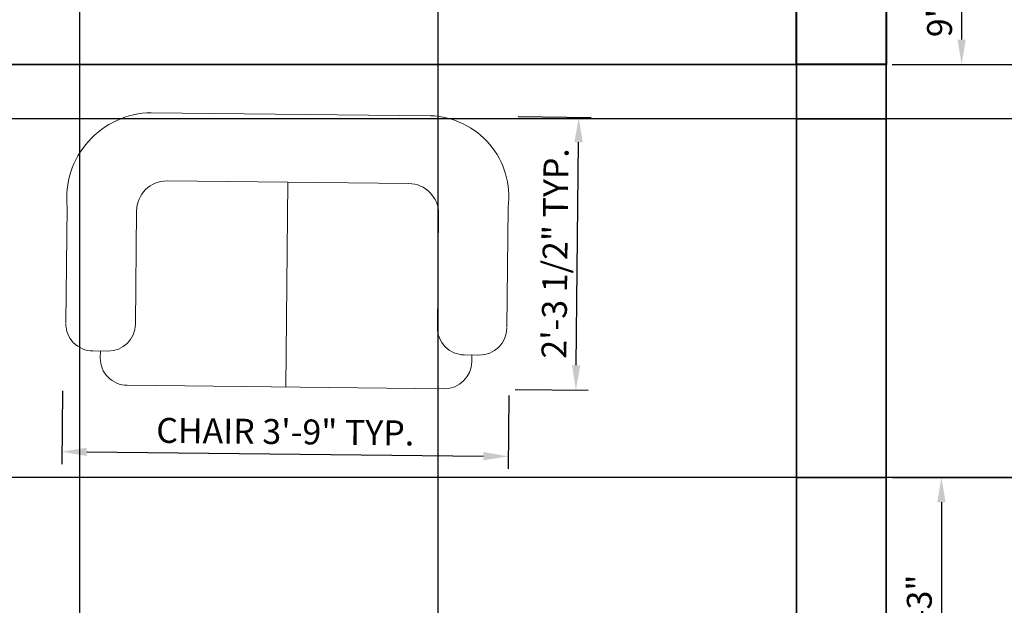
# Model space of a CAD drawing. Units: inches. Extents: x 1624 to 3956, y 1589 to 5028.
# Tile 7 of 16: x 2014 to 2112, y 2191 to 2250. Entities that reach past the tile are written whole.
import ezdxf

# ---------------------------------------------------------------- set-up
doc = ezdxf.new("R2010")
doc.units = ezdxf.units.IN
for name, color, linetype, lineweight in [('A-ANNO-DIMS', 2, 'Continuous', 13), ('A-COLS', 1, 'Continuous', 40), ('A-FURN', 8, 'Continuous', 18), ('A-WALL', 7, 'Continuous', 35)]:
    doc.layers.add(name, color=color, linetype=linetype, lineweight=lineweight)
doc.styles.get("Standard").update_dxf_attribs({"font": 'arial.ttf'})
doc.dimstyles.new('Copy of ISO-25', dxfattribs={"dimtxt": 2.5, "dimasz": 2.5, "dimexe": 1.25, "dimexo": 0.625, "dimtad": 1, "dimdec": 1, "dimlunit": 4, "dimtxsty": 'Standard', "dimcen": 2.5, "dimadec": 0, "dimazin": 0, "dimtfac": 1, "dimtdec": 1, "dimtmove": 0, "dimatfit": 3, "dimfxl": 1, "dimarcsym": 0})

# ---------------------------------------------------------------- blocks, each defined once
blk = doc.blocks.new('A$C6D011943')
for p, q in [((1.4484, 1.0893), (0.3319, 1.0893)), ((1.3639, 0.8177), (0.3983, 0.8177)), ((0.8811, 0.8177), (0.8811, 0)), ((0, 0.7091), (0, 0.2474)), ((1.7622, 0.2474), (1.7622, 0.7272)), ((0.2776, 0.697), (0.2776, 0.2444)), ((1.4846, 0.2444), (1.4846, 0.697)), ((0.1086, 0.1358), (0.169, 0.1358)), ((0.1388, 0.1086), (0.1388, 0.1358)), ((1.5932, 0.1358), (1.6536, 0.1358)), ((1.6475, 0.1358), (1.6234, 0.1358)), ((1.6234, 0.1086), (1.6234, 0.1358)), ((1.5148, 0), (0.2474, 0))]:
    blk.add_line(p, q)
for centre, radius, start, end in [((0.3394, 0.7478), 0.3416, 91.2564, 186.501), ((1.4409, 0.7658), 0.3236, 353.159, 88.6697), ((0.3983, 0.697), 0.1207, 90, 180), ((1.3639, 0.697), 0.1207, 0, 90), ((0.1086, 0.2444), 0.1086, 180, 270), ((0.169, 0.2444), 0.1086, 270, 0), ((1.5932, 0.2444), 0.1086, 180, 270), ((1.6536, 0.2444), 0.1086, 270, 0), ((0.2474, 0.1086), 0.1086, 180, 270), ((1.5148, 0.1086), 0.1086, 270, 0)]:
    blk.add_arc(centre, radius, start, end)
blk = doc.blocks.new('*D38')
at = {"layer": 'A-ANNO-DIMS', "color": 0, "lineweight": -2, "transparency": 16777216}
for p, q in [((2101.204, 2254.295), (2109.428, 2254.295)), ((2108.178, 2251.795), (2108.178, 2247.795)), ((2101.204, 2245.295), (2109.428, 2245.295))]:
    blk.add_line(p, q, dxfattribs=at)
at = {"layer": 'A-ANNO-DIMS', "color": 0, "transparency": 16777216}
for points in [[(2107.761, 2251.795), (2108.594, 2251.795), (2108.178, 2254.295)], [(2107.761, 2247.795), (2108.594, 2247.795), (2108.178, 2245.295)]]:
    blk.add_solid(points, dxfattribs=at)
at = {"layer": 'Defpoints', "color": 0, "transparency": 16777216}
for p in [(2100.579, 2254.295), (2100.579, 2245.295), (2108.178, 2245.295)]:
    blk.add_point(p, dxfattribs=at)
at = {"layer": 'A-ANNO-DIMS', "color": 0, "transparency": 16777216, "insert": (2106.276, 2249.795), "char_height": 2.5, "attachment_point": 5, "rotation": 90}
blk.add_mtext('9"', dxfattribs=at)
blk = doc.blocks.new('*D39')
at = {"layer": 'A-ANNO-DIMS', "color": 0, "lineweight": -2, "transparency": 16777216}
for p, q in [((2101.204, 2203.835), (2107.397, 2203.835)), ((2106.147, 2201.335), (2106.147, 2179.295)), ((2101.204, 2176.795), (2107.397, 2176.795))]:
    blk.add_line(p, q, dxfattribs=at)
at = {"layer": 'A-ANNO-DIMS', "color": 0, "transparency": 16777216}
for points in [[(2105.73, 2201.335), (2106.564, 2201.335), (2106.147, 2203.835)], [(2105.73, 2179.295), (2106.564, 2179.295), (2106.147, 2176.795)]]:
    blk.add_solid(points, dxfattribs=at)
at = {"layer": 'Defpoints', "color": 0, "transparency": 16777216}
for p in [(2100.579, 2203.835), (2100.579, 2176.795), (2106.147, 2176.795)]:
    blk.add_point(p, dxfattribs=at)
at = {"layer": 'A-ANNO-DIMS', "color": 0, "transparency": 16777216, "insert": (2104.245, 2190.315), "char_height": 2.5, "attachment_point": 5, "rotation": 90}
blk.add_mtext('2\'-3"', dxfattribs=at)
blk = doc.blocks.new('COLUMN-9x9')
for p, q in [((0, 0), (0, 9)), ((0, 9), (9, 9)), ((9, 9), (9, 0)), ((9, 0), (0, 0))]:
    blk.add_line(p, q)
blk = doc.blocks.new('*D52')
at = {"layer": 'A-ANNO-DIMS', "color": 0, "lineweight": -2, "transparency": 16777216}
for p, q in [((2017.817, 2212.527), (2017.739, 2205.174)), ((2062.676, 2212.049), (2062.598, 2204.695)), ((2020.252, 2206.397), (2060.111, 2205.972))]:
    blk.add_line(p, q, dxfattribs=at)
at = {"layer": 'A-ANNO-DIMS', "color": 0, "transparency": 16777216}
for points in [[(2020.256, 2206.813), (2020.247, 2205.98), (2017.752, 2206.423)], [(2060.116, 2206.388), (2060.107, 2205.555), (2062.611, 2205.945)]]:
    blk.add_solid(points, dxfattribs=at)
at = {"layer": 'Defpoints', "color": 0, "transparency": 16777216}
for p in [(2017.824, 2213.152), (2062.683, 2212.674), (2062.611, 2205.945)]:
    blk.add_point(p, dxfattribs=at)
at = {"layer": 'A-ANNO-DIMS', "color": 0, "transparency": 16777216, "insert": (2040.202, 2208.103), "char_height": 2.5, "attachment_point": 5, "rotation": 359.38916}
blk.add_mtext('CHAIR 3\'-9" TYP.', dxfattribs=at)
blk = doc.blocks.new('*D53')
at = {"layer": 'A-ANNO-DIMS', "color": 0, "lineweight": -2, "transparency": 16777216}
for p, q in [((2063.6, 2240.059), (2070.954, 2239.981)), ((2069.438, 2215.102), (2069.677, 2237.495)), ((2063.308, 2212.667), (2070.662, 2212.589))]:
    blk.add_line(p, q, dxfattribs=at)
at = {"layer": 'A-ANNO-DIMS', "color": 0, "transparency": 16777216}
for points in [[(2069.26, 2237.499), (2070.094, 2237.49), (2069.704, 2239.994)], [(2069.022, 2215.107), (2069.855, 2215.098), (2069.412, 2212.602)]]:
    blk.add_solid(points, dxfattribs=at)
at = {"layer": 'Defpoints', "color": 0, "transparency": 16777216}
for p in [(2062.975, 2240.066), (2069.704, 2239.994), (2062.683, 2212.674)]:
    blk.add_point(p, dxfattribs=at)
at = {"layer": 'A-ANNO-DIMS', "color": 0, "transparency": 16777216, "insert": (2067.639, 2226.319), "char_height": 2.5, "attachment_point": 5, "rotation": 89.38916}
blk.add_mtext('2\'-3 1/2" TYP.', dxfattribs=at)
blk = doc.blocks.new('*D80')
at = {"layer": 'A-ANNO-DIMS', "color": 0, "lineweight": -2, "transparency": 16777216}
for p, q in [((2101.204, 2245.295), (2217.629, 2245.295)), ((2216.379, 2206.335), (2216.379, 2242.795)), ((2101.204, 2203.835), (2217.629, 2203.835))]:
    blk.add_line(p, q, dxfattribs=at)
at = {"layer": 'A-ANNO-DIMS', "color": 0, "transparency": 16777216}
for points in [[(2215.963, 2242.795), (2216.796, 2242.795), (2216.379, 2245.295)], [(2215.963, 2206.335), (2216.796, 2206.335), (2216.379, 2203.835)]]:
    blk.add_solid(points, dxfattribs=at)
at = {"layer": 'Defpoints', "color": 0, "transparency": 16777216}
for p in [(2100.579, 2245.295), (2216.379, 2245.295), (2100.579, 2203.835)]:
    blk.add_point(p, dxfattribs=at)
at = {"layer": 'A-ANNO-DIMS', "color": 0, "transparency": 16777216, "insert": (2214.461, 2224.565), "char_height": 2.5, "attachment_point": 5, "rotation": 90}
blk.add_mtext('3\'-5 1/2"', dxfattribs=at)
blk = doc.blocks.new('*D90')
at = {"layer": 'A-ANNO-DIMS', "color": 0, "lineweight": -2, "transparency": 16777216}
for p, q in [((2019.579, 1941.92), (2019.579, 2612.845)), ((2055.579, 1941.92), (2055.579, 2612.845)), ((2022.079, 2611.595), (2053.079, 2611.595))]:
    blk.add_line(p, q, dxfattribs=at)
at = {"layer": 'A-ANNO-DIMS', "color": 0, "transparency": 16777216}
for points in [[(2022.079, 2612.011), (2022.079, 2611.178), (2019.579, 2611.595)], [(2053.079, 2612.011), (2053.079, 2611.178), (2055.579, 2611.595)]]:
    blk.add_solid(points, dxfattribs=at)
at = {"layer": 'Defpoints', "color": 0, "transparency": 16777216}
for p in [(2055.579, 2611.595), (2019.579, 1941.295), (2055.579, 1941.295)]:
    blk.add_point(p, dxfattribs=at)
at = {"layer": 'A-ANNO-DIMS', "color": 0, "transparency": 16777216, "insert": (2037.579, 2613.497), "char_height": 2.5, "attachment_point": 5}
blk.add_mtext('3\'-0"', dxfattribs=at)
blk = doc.blocks.new('*D95')
at = {"layer": 'A-ANNO-DIMS', "color": 0, "lineweight": -2, "transparency": 16777216}
for p, q in [((1870.181, 2239.871), (2217.629, 2239.871)), ((2216.379, 2206.371), (2216.379, 2237.371)), ((1870.181, 2203.871), (2217.629, 2203.871))]:
    blk.add_line(p, q, dxfattribs=at)
at = {"layer": 'A-ANNO-DIMS', "color": 0, "transparency": 16777216}
for points in [[(2215.963, 2237.371), (2216.796, 2237.371), (2216.379, 2239.871)], [(2215.963, 2206.371), (2216.796, 2206.371), (2216.379, 2203.871)]]:
    blk.add_solid(points, dxfattribs=at)
at = {"layer": 'Defpoints', "color": 0, "transparency": 16777216}
for p in [(1869.556, 2239.871), (2216.379, 2239.871), (1869.556, 2203.871)]:
    blk.add_point(p, dxfattribs=at)
at = {"layer": 'A-ANNO-DIMS', "color": 0, "transparency": 16777216, "insert": (2214.477, 2221.871), "char_height": 2.5, "attachment_point": 5, "rotation": 90}
blk.add_mtext('3\'-0"', dxfattribs=at)
blk = doc.blocks.new('*D98')
at = {"layer": 'A-ANNO-DIMS', "color": 0, "lineweight": -2, "transparency": 16777216}
for p, q in [((2090.954, 2245.295), (1628.859, 2245.295)), ((1630.109, 2079.795), (1630.109, 2242.795)), ((2090.954, 2077.295), (1628.859, 2077.295))]:
    blk.add_line(p, q, dxfattribs=at)
at = {"layer": 'A-ANNO-DIMS', "color": 0, "transparency": 16777216}
for points in [[(1629.692, 2242.795), (1630.525, 2242.795), (1630.109, 2245.295)], [(1629.692, 2079.795), (1630.525, 2079.795), (1630.109, 2077.295)]]:
    blk.add_solid(points, dxfattribs=at)
at = {"layer": 'Defpoints', "color": 0, "transparency": 16777216}
for p in [(1630.109, 2245.295), (2091.579, 2245.295), (2091.579, 2077.295)]:
    blk.add_point(p, dxfattribs=at)
at = {"layer": 'A-ANNO-DIMS', "color": 0, "transparency": 16777216, "insert": (1628.207, 2161.295), "char_height": 2.5, "attachment_point": 5, "rotation": 90}
blk.add_mtext('14\'-0"', dxfattribs=at)

msp = doc.modelspace()

# ---------------------------------------------------------------- linework, layer by layer
at = {"layer": 'A-WALL'}
for p, q in [((2100.579, 2254.295), (2100.579, 2161.295)), ((2100.579, 2245.295), (2100.579, 2254.295)), ((2091.579, 2245.295), (1960.579, 2245.295)), ((2091.579, 2077.295), (2091.579, 2245.295)), ((2091.579, 2245.295), (2091.579, 2240.795)), ((2100.579, 2245.295), (2100.579, 2077.295)), ((2100.579, 2245.295), (2100.579, 2239.835)), ((2091.579, 2240.795), (2091.579, 2204.795)), ((2100.579, 2239.835), (2091.579, 2239.835)), ((2091.579, 2239.835), (2091.579, 2203.835)), ((2091.579, 2204.795), (2091.579, 2176.795)), ((2091.579, 2203.835), (2100.579, 2203.835))]:
    msp.add_line(p, q, dxfattribs=at)

# ---------------------------------------------------------------- block references
at = {"layer": 'A-COLS', "rotation": 270.0000000000029}
msp.add_blockref('COLUMN-9x9', (2091.579, 2254.295), dxfattribs=at)
at = {"layer": 'A-FURN', "xscale": 25.14761962403201, "yscale": 25.14761962403201, "zscale": 25.14761962403201, "rotation": 359.3891645815014}
msp.add_blockref('A$C6D011943', (2018.097, 2213.149), dxfattribs=at)

# ---------------------------------------------------------------- dimensions: what is measured, and where the dimension line sits
at = {"layer": 'A-ANNO-DIMS'}
dim = msp.add_linear_dim(base=(2055.579, 2611.595), p1=(2019.579, 1941.295), p2=(2055.579, 1941.295), dimstyle='Copy of ISO-25', override={"dimdec": 1, "dimlfac": 1, "dimrnd": 0, "dimzin": 1, "dimdsep": 46, "dimlunit": 4, "dimfrac": 2}, dxfattribs=at)
dim.commit()
dim.dimension.update_dxf_attribs({"geometry": '*D90', "text_midpoint": (2037.579, 2613.497)})
for base, p1, p2, override, picture, middle in [((2108.178, 2245.295), (2100.579, 2254.295), (2100.579, 2245.295), {"dimclrd": 0, "dimclre": 0, "dimclrt": 0}, '*D38', (2106.276, 2249.795)), ((1630.109, 2245.295), (2091.579, 2077.295), (2091.579, 2245.295), {"dimdec": 1, "dimlfac": 1, "dimrnd": 0, "dimzin": 1, "dimdsep": 46, "dimlunit": 4, "dimfrac": 2}, '*D98', (1628.207, 2161.295)), ((2216.379, 2245.295), (2100.579, 2203.835), (2100.579, 2245.295), {"dimdec": 1, "dimlfac": 1, "dimrnd": 0, "dimzin": 1, "dimdsep": 46, "dimlunit": 4, "dimfrac": 2}, '*D80', (2214.461, 2224.565)), ((2216.379, 2239.871), (1869.556, 2203.871), (1869.556, 2239.871), {"dimdec": 1, "dimlfac": 1, "dimrnd": 0, "dimzin": 1, "dimdsep": 46, "dimlunit": 4, "dimfrac": 2}, '*D95', (2214.477, 2221.871)), ((2106.147, 2176.795), (2100.579, 2203.835), (2100.579, 2176.795), {"dimclrd": 0, "dimclre": 0, "dimclrt": 0}, '*D39', (2104.245, 2190.315))]:
    dim = msp.add_linear_dim(base=base, p1=p1, p2=p2, angle=90, dimstyle='Copy of ISO-25', override=override, dxfattribs=at)
    dim.commit()
    dim.dimension.update_dxf_attribs({"geometry": picture, "text_midpoint": middle})
for base, p1, p2, angle, text, picture, middle in [((2069.704, 2239.994), (2062.683, 2212.674), (2062.975, 2240.066), 89.38916, '<> TYP.', '*D53', (2067.639, 2226.319)), ((2062.611, 2205.945), (2017.824, 2213.152), (2062.683, 2212.674), 359.38916, 'CHAIR <> TYP.', '*D52', (2040.202, 2208.103))]:
    dim = msp.add_linear_dim(base=base, p1=p1, p2=p2, angle=angle, text=text, dimstyle='Copy of ISO-25', override={"dimdec": 1, "dimlfac": 1, "dimrnd": 0, "dimzin": 1, "dimdsep": 46, "dimlunit": 4, "dimfrac": 2}, dxfattribs=at)
    dim.commit()
    dim.dimension.update_dxf_attribs({"geometry": picture, "text_midpoint": middle})

doc.saveas('drawing.dxf')
